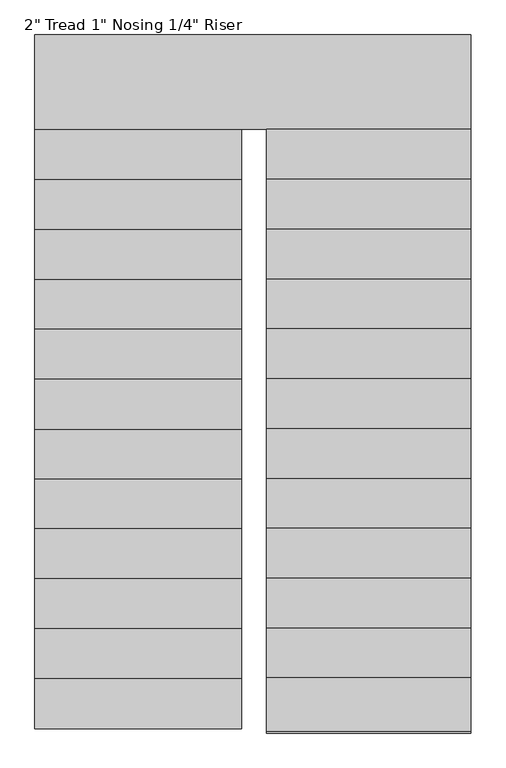
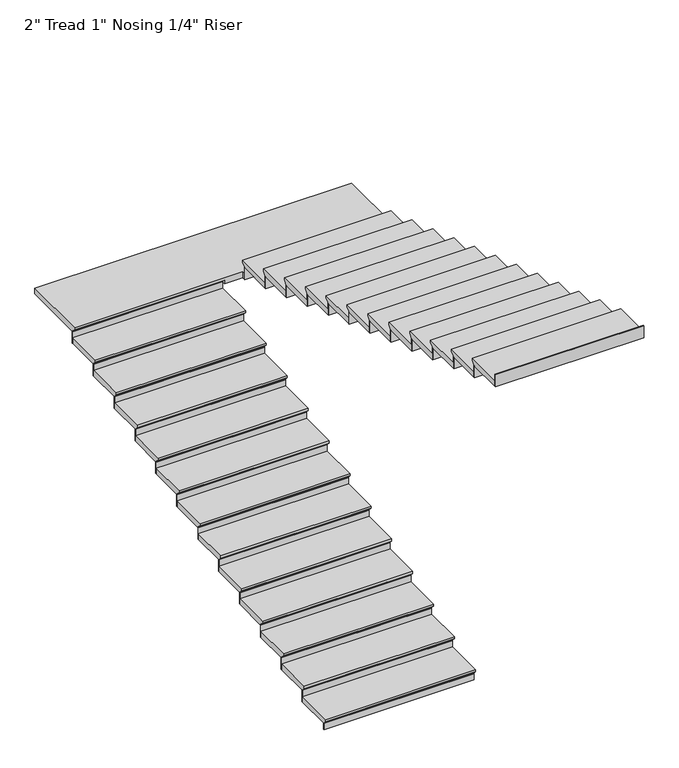
"""IFC4 building model written with IfcOpenShell, lengths in millimetres: stair flight geometry."""

from ifc_helpers import new_model, si_unit, origin, place, context, project, spatial, faceted_brep, source, transform, mapped, element, save


def stair_flight_b14bcda7(model_context):
    return source(origin(), model_context, "Body", "Brep", [
        faceted_brep([(-2593.7381751, -9955.5916506, 6182.4576923), (-2593.7381751, -9955.5916506, 6201.5076923), (-3857.687215, -9955.5916506, 6201.5076923), (-3857.687215, -9955.5916506, 6182.4576923), (-2593.7381751, -9930.1916506, 6157.0576923), (-3857.687215, -9930.1916506, 6157.0576923), (-2593.7381751, -9619.0416506, 6201.5076923), (-3857.687215, -9619.0416506, 6201.5076923), (-3857.687215, -9930.1916506, 6150.7076923), (-3857.687215, -9619.0416506, 6150.7076923), (-2593.7381751, -9619.0416506, 6150.7076923), (-2593.7381751, -9930.1916506, 6150.7076923)], [[[0, 1, 2, 3]], [[4, 0, 3, 5]], [[2, 1, 6, 7]], [[8, 9, 10, 11]], [[2, 7, 9, 8, 5, 3]], [[8, 11, 4, 5]], [[6, 1, 0, 4, 11, 10]], [[7, 6, 10, 9]]]),
        faceted_brep([(-2593.7381751, -9930.1916506, 6150.7076923), (-2593.7381751, -9930.1916506, 6096.0), (-2593.7381751, -9923.8416506, 6096.0), (-2593.7381751, -9923.8416506, 6150.7076923), (-3857.687215, -9930.1916506, 6150.7076923), (-3857.687215, -9923.8416506, 6150.7076923), (-3857.687215, -9923.8416506, 6096.0), (-3857.687215, -9930.1916506, 6096.0)], [[[0, 1, 2, 3]], [[4, 5, 6, 7]], [[1, 0, 4, 7]], [[2, 1, 7, 6]], [[3, 2, 6, 5]], [[0, 3, 5, 4]]]),
        faceted_brep([(-2593.7381751, -9619.0416506, 6256.2153846), (-2593.7381751, -9619.0416506, 6150.7076923), (-2593.7381751, -9612.6916506, 6150.7076923), (-2593.7381751, -9612.6916506, 6256.2153846), (-3857.687215, -9619.0416506, 6256.2153846), (-3857.687215, -9612.6916506, 6256.2153846), (-3857.687215, -9612.6916506, 6150.7076923), (-3857.687215, -9619.0416506, 6150.7076923)], [[[0, 1, 2, 3]], [[4, 5, 6, 7]], [[1, 0, 4, 7]], [[2, 1, 7, 6]], [[3, 2, 6, 5]], [[0, 3, 5, 4]]]),
        faceted_brep([(-3857.687215, -9644.4416506, 6307.0153846), (-2593.7381751, -9644.4416506, 6307.0153846), (-2593.7381751, -9314.2416506, 6307.0153846), (-3857.687215, -9314.2416506, 6307.0153846), (-3857.687215, -9619.0416506, 6256.2153846), (-3857.687215, -9314.2416506, 6256.2153846), (-2593.7381751, -9314.2416506, 6256.2153846), (-2593.7381751, -9619.0416506, 6256.2153846), (-3857.687215, -9619.0416506, 6262.5653846), (-3857.687215, -9644.4416506, 6287.9653846), (-2593.7381751, -9619.0416506, 6262.5653846), (-2593.7381751, -9644.4416506, 6287.9653846)], [[[0, 1, 2, 3]], [[4, 5, 6, 7]], [[0, 3, 5, 4, 8, 9]], [[4, 7, 10, 8]], [[2, 1, 11, 10, 7, 6]], [[3, 2, 6, 5]], [[11, 1, 0, 9]], [[10, 11, 9, 8]]]),
        faceted_brep([(-2593.7381751, -9314.2416506, 6361.7230769), (-2593.7381751, -9314.2416506, 6256.2153846), (-2593.7381751, -9307.8916506, 6256.2153846), (-2593.7381751, -9307.8916506, 6361.7230769), (-3857.687215, -9314.2416506, 6361.7230769), (-3857.687215, -9307.8916506, 6361.7230769), (-3857.687215, -9307.8916506, 6256.2153846), (-3857.687215, -9314.2416506, 6256.2153846)], [[[0, 1, 2, 3]], [[4, 5, 6, 7]], [[1, 0, 4, 7]], [[2, 1, 7, 6]], [[3, 2, 6, 5]], [[0, 3, 5, 4]]]),
        faceted_brep([(-3857.687215, -9339.6416506, 6412.5230769), (-2593.7381751, -9339.6416506, 6412.5230769), (-2593.7381751, -9009.4416506, 6412.5230769), (-3857.687215, -9009.4416506, 6412.5230769), (-3857.687215, -9314.2416506, 6361.7230769), (-3857.687215, -9009.4416506, 6361.7230769), (-2593.7381751, -9009.4416506, 6361.7230769), (-2593.7381751, -9314.2416506, 6361.7230769), (-3857.687215, -9314.2416506, 6368.0730769), (-3857.687215, -9339.6416506, 6393.4730769), (-2593.7381751, -9314.2416506, 6368.0730769), (-2593.7381751, -9339.6416506, 6393.4730769)], [[[0, 1, 2, 3]], [[4, 5, 6, 7]], [[0, 3, 5, 4, 8, 9]], [[4, 7, 10, 8]], [[2, 1, 11, 10, 7, 6]], [[3, 2, 6, 5]], [[11, 1, 0, 9]], [[10, 11, 9, 8]]]),
        faceted_brep([(-2593.7381751, -9009.4416506, 6467.2307692), (-2593.7381751, -9009.4416506, 6361.7230769), (-2593.7381751, -9003.0916506, 6361.7230769), (-2593.7381751, -9003.0916506, 6467.2307692), (-3857.687215, -9009.4416506, 6467.2307692), (-3857.687215, -9003.0916506, 6467.2307692), (-3857.687215, -9003.0916506, 6361.7230769), (-3857.687215, -9009.4416506, 6361.7230769)], [[[0, 1, 2, 3]], [[4, 5, 6, 7]], [[1, 0, 4, 7]], [[2, 1, 7, 6]], [[3, 2, 6, 5]], [[0, 3, 5, 4]]]),
        faceted_brep([(-3857.687215, -9034.8416506, 6518.0307692), (-2593.7381751, -9034.8416506, 6518.0307692), (-2593.7381751, -8704.6416506, 6518.0307692), (-3857.687215, -8704.6416506, 6518.0307692), (-3857.687215, -9009.4416506, 6467.2307692), (-3857.687215, -8704.6416506, 6467.2307692), (-2593.7381751, -8704.6416506, 6467.2307692), (-2593.7381751, -9009.4416506, 6467.2307692), (-3857.687215, -9009.4416506, 6473.5807692), (-3857.687215, -9034.8416506, 6498.9807692), (-2593.7381751, -9009.4416506, 6473.5807692), (-2593.7381751, -9034.8416506, 6498.9807692)], [[[0, 1, 2, 3]], [[4, 5, 6, 7]], [[0, 3, 5, 4, 8, 9]], [[4, 7, 10, 8]], [[2, 1, 11, 10, 7, 6]], [[3, 2, 6, 5]], [[11, 1, 0, 9]], [[10, 11, 9, 8]]]),
        faceted_brep([(-2593.7381751, -8704.6416506, 6572.7384615), (-2593.7381751, -8704.6416506, 6467.2307692), (-2593.7381751, -8698.2916506, 6467.2307692), (-2593.7381751, -8698.2916506, 6572.7384615), (-3857.687215, -8704.6416506, 6572.7384615), (-3857.687215, -8698.2916506, 6572.7384615), (-3857.687215, -8698.2916506, 6467.2307692), (-3857.687215, -8704.6416506, 6467.2307692)], [[[0, 1, 2, 3]], [[4, 5, 6, 7]], [[1, 0, 4, 7]], [[2, 1, 7, 6]], [[3, 2, 6, 5]], [[0, 3, 5, 4]]]),
        faceted_brep([(-3857.687215, -8730.0416506, 6623.5384615), (-2593.7381751, -8730.0416506, 6623.5384615), (-2593.7381751, -8399.8416506, 6623.5384615), (-3857.687215, -8399.8416506, 6623.5384615), (-3857.687215, -8704.6416506, 6572.7384615), (-3857.687215, -8399.8416506, 6572.7384615), (-2593.7381751, -8399.8416506, 6572.7384615), (-2593.7381751, -8704.6416506, 6572.7384615), (-3857.687215, -8704.6416506, 6579.0884615), (-3857.687215, -8730.0416506, 6604.4884615), (-2593.7381751, -8704.6416506, 6579.0884615), (-2593.7381751, -8730.0416506, 6604.4884615)], [[[0, 1, 2, 3]], [[4, 5, 6, 7]], [[0, 3, 5, 4, 8, 9]], [[4, 7, 10, 8]], [[2, 1, 11, 10, 7, 6]], [[3, 2, 6, 5]], [[11, 1, 0, 9]], [[10, 11, 9, 8]]]),
        faceted_brep([(-2593.7381751, -8399.8416506, 6678.2461538), (-2593.7381751, -8399.8416506, 6572.7384615), (-2593.7381751, -8393.4916506, 6572.7384615), (-2593.7381751, -8393.4916506, 6678.2461538), (-3857.687215, -8399.8416506, 6678.2461538), (-3857.687215, -8393.4916506, 6678.2461538), (-3857.687215, -8393.4916506, 6572.7384615), (-3857.687215, -8399.8416506, 6572.7384615)], [[[0, 1, 2, 3]], [[4, 5, 6, 7]], [[1, 0, 4, 7]], [[2, 1, 7, 6]], [[3, 2, 6, 5]], [[0, 3, 5, 4]]]),
        faceted_brep([(-3857.687215, -8425.2416506, 6729.0461538), (-2593.7381751, -8425.2416506, 6729.0461538), (-2593.7381751, -8098.2166506, 6729.0461538), (-3857.687215, -8098.2166506, 6729.0461538), (-3857.687215, -8399.8416506, 6678.2461538), (-3857.687215, -8098.2166506, 6678.2461538), (-2593.7381751, -8098.2166506, 6678.2461538), (-2593.7381751, -8399.8416506, 6678.2461538), (-3857.687215, -8399.8416506, 6684.5961538), (-3857.687215, -8425.2416506, 6709.9961538), (-2593.7381751, -8399.8416506, 6684.5961538), (-2593.7381751, -8425.2416506, 6709.9961538)], [[[0, 1, 2, 3]], [[4, 5, 6, 7]], [[0, 3, 5, 4, 8, 9]], [[4, 7, 10, 8]], [[2, 1, 11, 10, 7, 6]], [[3, 2, 6, 5]], [[11, 1, 0, 9]], [[10, 11, 9, 8]]]),
        faceted_brep([(-2593.7381751, -8098.2166506, 6783.7538462), (-2593.7381751, -8098.2166506, 6678.2461538), (-2593.7381751, -8091.8666506, 6678.2461538), (-2593.7381751, -8091.8666506, 6783.7538462), (-3857.687215, -8098.2166506, 6783.7538462), (-3857.687215, -8091.8666506, 6783.7538462), (-3857.687215, -8091.8666506, 6678.2461538), (-3857.687215, -8098.2166506, 6678.2461538)], [[[0, 1, 2, 3]], [[4, 5, 6, 7]], [[1, 0, 4, 7]], [[2, 1, 7, 6]], [[3, 2, 6, 5]], [[0, 3, 5, 4]]]),
        faceted_brep([(-3857.687215, -8123.6166506, 6834.5538462), (-2593.7381751, -8123.6166506, 6834.5538462), (-2593.7381751, -7790.2416506, 6834.5538462), (-3857.687215, -7790.2416506, 6834.5538462), (-3857.687215, -8098.2166506, 6783.7538462), (-3857.687215, -7790.2416506, 6783.7538462), (-2593.7381751, -7790.2416506, 6783.7538462), (-2593.7381751, -8098.2166506, 6783.7538462), (-3857.687215, -8098.2166506, 6790.1038462), (-3857.687215, -8123.6166506, 6815.5038462), (-2593.7381751, -8098.2166506, 6790.1038462), (-2593.7381751, -8123.6166506, 6815.5038462)], [[[0, 1, 2, 3]], [[4, 5, 6, 7]], [[0, 3, 5, 4, 8, 9]], [[4, 7, 10, 8]], [[2, 1, 11, 10, 7, 6]], [[3, 2, 6, 5]], [[11, 1, 0, 9]], [[10, 11, 9, 8]]]),
        faceted_brep([(-2593.7381751, -7790.2416506, 6889.2615385), (-2593.7381751, -7790.2416506, 6783.7538462), (-2593.7381751, -7783.8916506, 6783.7538462), (-2593.7381751, -7783.8916506, 6889.2615385), (-3857.687215, -7790.2416506, 6889.2615385), (-3857.687215, -7783.8916506, 6889.2615385), (-3857.687215, -7783.8916506, 6783.7538462), (-3857.687215, -7790.2416506, 6783.7538462)], [[[0, 1, 2, 3]], [[4, 5, 6, 7]], [[1, 0, 4, 7]], [[2, 1, 7, 6]], [[3, 2, 6, 5]], [[0, 3, 5, 4]]]),
        faceted_brep([(-3857.687215, -7815.6416506, 6940.0615385), (-2593.7381751, -7815.6416506, 6940.0615385), (-2593.7381751, -7485.4416506, 6940.0615385), (-3857.687215, -7485.4416506, 6940.0615385), (-3857.687215, -7790.2416506, 6889.2615385), (-3857.687215, -7485.4416506, 6889.2615385), (-2593.7381751, -7485.4416506, 6889.2615385), (-2593.7381751, -7790.2416506, 6889.2615385), (-3857.687215, -7790.2416506, 6895.6115385), (-3857.687215, -7815.6416506, 6921.0115385), (-2593.7381751, -7790.2416506, 6895.6115385), (-2593.7381751, -7815.6416506, 6921.0115385)], [[[0, 1, 2, 3]], [[4, 5, 6, 7]], [[0, 3, 5, 4, 8, 9]], [[4, 7, 10, 8]], [[2, 1, 11, 10, 7, 6]], [[3, 2, 6, 5]], [[11, 1, 0, 9]], [[10, 11, 9, 8]]]),
        faceted_brep([(-2593.7381751, -7485.4416506, 6994.7692308), (-2593.7381751, -7485.4416506, 6889.2615385), (-2593.7381751, -7479.0916506, 6889.2615385), (-2593.7381751, -7479.0916506, 6994.7692308), (-3857.687215, -7485.4416506, 6994.7692308), (-3857.687215, -7479.0916506, 6994.7692308), (-3857.687215, -7479.0916506, 6889.2615385), (-3857.687215, -7485.4416506, 6889.2615385)], [[[0, 1, 2, 3]], [[4, 5, 6, 7]], [[1, 0, 4, 7]], [[2, 1, 7, 6]], [[3, 2, 6, 5]], [[0, 3, 5, 4]]]),
        faceted_brep([(-3857.687215, -7510.8416506, 7045.5692308), (-2593.7381751, -7510.8416506, 7045.5692308), (-2593.7381751, -7180.6416506, 7045.5692308), (-3857.687215, -7180.6416506, 7045.5692308), (-3857.687215, -7485.4416506, 6994.7692308), (-3857.687215, -7180.6416506, 6994.7692308), (-2593.7381751, -7180.6416506, 6994.7692308), (-2593.7381751, -7485.4416506, 6994.7692308), (-3857.687215, -7485.4416506, 7001.1192308), (-3857.687215, -7510.8416506, 7026.5192308), (-2593.7381751, -7485.4416506, 7001.1192308), (-2593.7381751, -7510.8416506, 7026.5192308)], [[[0, 1, 2, 3]], [[4, 5, 6, 7]], [[0, 3, 5, 4, 8, 9]], [[4, 7, 10, 8]], [[2, 1, 11, 10, 7, 6]], [[3, 2, 6, 5]], [[11, 1, 0, 9]], [[10, 11, 9, 8]]]),
        faceted_brep([(-2593.7381751, -7180.6416506, 7100.2769231), (-2593.7381751, -7180.6416506, 6994.7692308), (-2593.7381751, -7174.2916506, 6994.7692308), (-2593.7381751, -7174.2916506, 7100.2769231), (-3857.687215, -7180.6416506, 7100.2769231), (-3857.687215, -7174.2916506, 7100.2769231), (-3857.687215, -7174.2916506, 6994.7692308), (-3857.687215, -7180.6416506, 6994.7692308)], [[[0, 1, 2, 3]], [[4, 5, 6, 7]], [[1, 0, 4, 7]], [[2, 1, 7, 6]], [[3, 2, 6, 5]], [[0, 3, 5, 4]]]),
        faceted_brep([(-3857.687215, -7206.0416506, 7151.0769231), (-2593.7381751, -7206.0416506, 7151.0769231), (-2593.7381751, -6875.8416506, 7151.0769231), (-3857.687215, -6875.8416506, 7151.0769231), (-3857.687215, -7180.6416506, 7100.2769231), (-3857.687215, -6875.8416506, 7100.2769231), (-2593.7381751, -6875.8416506, 7100.2769231), (-2593.7381751, -7180.6416506, 7100.2769231), (-3857.687215, -7180.6416506, 7106.6269231), (-3857.687215, -7206.0416506, 7132.0269231), (-2593.7381751, -7180.6416506, 7106.6269231), (-2593.7381751, -7206.0416506, 7132.0269231)], [[[0, 1, 2, 3]], [[4, 5, 6, 7]], [[0, 3, 5, 4, 8, 9]], [[4, 7, 10, 8]], [[2, 1, 11, 10, 7, 6]], [[3, 2, 6, 5]], [[11, 1, 0, 9]], [[10, 11, 9, 8]]]),
        faceted_brep([(-2593.7381751, -6875.8416506, 7205.7846154), (-2593.7381751, -6875.8416506, 7100.2769231), (-2593.7381751, -6869.4916506, 7100.2769231), (-2593.7381751, -6869.4916506, 7205.7846154), (-3857.687215, -6875.8416506, 7205.7846154), (-3857.687215, -6869.4916506, 7205.7846154), (-3857.687215, -6869.4916506, 7100.2769231), (-3857.687215, -6875.8416506, 7100.2769231)], [[[0, 1, 2, 3]], [[4, 5, 6, 7]], [[1, 0, 4, 7]], [[2, 1, 7, 6]], [[3, 2, 6, 5]], [[0, 3, 5, 4]]]),
        faceted_brep([(-3857.687215, -6901.2416506, 7256.5846154), (-2593.7381751, -6901.2416506, 7256.5846154), (-2593.7381751, -6571.0416506, 7256.5846154), (-3857.687215, -6571.0416506, 7256.5846154), (-3857.687215, -6875.8416506, 7205.7846154), (-3857.687215, -6571.0416506, 7205.7846154), (-2593.7381751, -6571.0416506, 7205.7846154), (-2593.7381751, -6875.8416506, 7205.7846154), (-3857.687215, -6875.8416506, 7212.1346154), (-3857.687215, -6901.2416506, 7237.5346154), (-2593.7381751, -6875.8416506, 7212.1346154), (-2593.7381751, -6901.2416506, 7237.5346154)], [[[0, 1, 2, 3]], [[4, 5, 6, 7]], [[0, 3, 5, 4, 8, 9]], [[4, 7, 10, 8]], [[2, 1, 11, 10, 7, 6]], [[3, 2, 6, 5]], [[11, 1, 0, 9]], [[10, 11, 9, 8]]]),
        faceted_brep([(-2593.7381751, -6571.0416506, 7311.2923077), (-2593.7381751, -6571.0416506, 7205.7846154), (-2593.7381751, -6564.6916506, 7205.7846154), (-2593.7381751, -6564.6916506, 7311.2923077), (-3857.687215, -6571.0416506, 7311.2923077), (-3857.687215, -6564.6916506, 7311.2923077), (-3857.687215, -6564.6916506, 7205.7846154), (-3857.687215, -6571.0416506, 7205.7846154)], [[[0, 1, 2, 3]], [[4, 5, 6, 7]], [[1, 0, 4, 7]], [[2, 1, 7, 6]], [[3, 2, 6, 5]], [[0, 3, 5, 4]]]),
        faceted_brep([(-3857.687215, -6596.4416506, 7362.0923077), (-2593.7381751, -6596.4416506, 7362.0923077), (-2593.7381751, -6266.2416506, 7362.0923077), (-3857.687215, -6266.2416506, 7362.0923077), (-3857.687215, -6571.0416506, 7311.2923077), (-3857.687215, -6266.2416506, 7311.2923077), (-2593.7381751, -6266.2416506, 7311.2923077), (-2593.7381751, -6571.0416506, 7311.2923077), (-3857.687215, -6571.0416506, 7317.6423077), (-3857.687215, -6596.4416506, 7343.0423077), (-2593.7381751, -6571.0416506, 7317.6423077), (-2593.7381751, -6596.4416506, 7343.0423077)], [[[0, 1, 2, 3]], [[4, 5, 6, 7]], [[0, 3, 5, 4, 8, 9]], [[4, 7, 10, 8]], [[2, 1, 11, 10, 7, 6]], [[3, 2, 6, 5]], [[11, 1, 0, 9]], [[10, 11, 9, 8]]]),
        faceted_brep([(-2593.7381751, -6266.2416506, 7416.8), (-2593.7381751, -6266.2416506, 7311.2923077), (-2593.7381751, -6259.8916506, 7311.2923077), (-2593.7381751, -6259.8916506, 7416.8), (-3857.687215, -6266.2416506, 7416.8), (-3857.687215, -6259.8916506, 7416.8), (-3857.687215, -6259.8916506, 7311.2923077), (-3857.687215, -6266.2416506, 7311.2923077)], [[[0, 1, 2, 3]], [[4, 5, 6, 7]], [[1, 0, 4, 7]], [[2, 1, 7, 6]], [[3, 2, 6, 5]], [[0, 3, 5, 4]]]),
        faceted_brep([(-1190.687215, -6317.0416506, 7467.6), (-1190.687215, -5713.7916506, 7467.6), (-3857.687215, -5713.7916506, 7467.6), (-3857.687215, -6291.6416506, 7467.6), (-2441.3381751, -6291.6416506, 7467.6), (-2441.3381751, -6317.0416506, 7467.6), (-1190.687215, -5713.7916506, 7416.8), (-1190.687215, -6317.0416506, 7416.8), (-2441.3381751, -6317.0416506, 7416.8), (-2441.3381751, -6291.6416506, 7416.8), (-2593.7381751, -6291.6416506, 7416.8), (-2593.7381751, -6266.2416506, 7416.8), (-3857.687215, -6266.2416506, 7416.8), (-3857.687215, -5713.7916506, 7416.8), (-3857.687215, -6266.2416506, 7423.15), (-3857.687215, -6291.6416506, 7448.55), (-2593.7381751, -6266.2416506, 7423.15), (-2593.7381751, -6291.6416506, 7448.55)], [[[0, 1, 2, 3, 4, 5]], [[6, 7, 8, 9, 10, 11, 12, 13]], [[1, 0, 7, 6]], [[2, 1, 6, 13]], [[3, 2, 13, 12, 14, 15]], [[12, 11, 16, 14]], [[11, 10, 17, 16]], [[4, 3, 15, 17, 10, 9]], [[5, 4, 9, 8]], [[0, 5, 8, 7]], [[15, 14, 16, 17]]]),
        faceted_brep([(-2441.3381751, -6317.0416506, 7522.3076923), (-2441.3381751, -6317.0416506, 7416.8), (-2441.3381751, -6323.3916506, 7416.8), (-2441.3381751, -6323.3916506, 7522.3076923), (-1190.687215, -6317.0416506, 7522.3076923), (-1190.687215, -6323.3916506, 7522.3076923), (-1190.687215, -6323.3916506, 7416.8), (-1190.687215, -6317.0416506, 7416.8)], [[[0, 1, 2, 3]], [[4, 5, 6, 7]], [[1, 0, 4, 7]], [[2, 1, 7, 6]], [[3, 2, 6, 5]], [[0, 3, 5, 4]]]),
        faceted_brep([(-1190.687215, -6291.6416506, 7573.1076923), (-2441.3381751, -6291.6416506, 7573.1076923), (-2441.3381751, -6621.8416506, 7573.1076923), (-1190.687215, -6621.8416506, 7573.1076923), (-1190.687215, -6317.0416506, 7522.3076923), (-1190.687215, -6621.8416506, 7522.3076923), (-2441.3381751, -6621.8416506, 7522.3076923), (-2441.3381751, -6317.0416506, 7522.3076923), (-1190.687215, -6317.0416506, 7528.6576923), (-1190.687215, -6291.6416506, 7554.0576923), (-2441.3381751, -6317.0416506, 7528.6576923), (-2441.3381751, -6291.6416506, 7554.0576923)], [[[0, 1, 2, 3]], [[4, 5, 6, 7]], [[0, 3, 5, 4, 8, 9]], [[4, 7, 10, 8]], [[2, 1, 11, 10, 7, 6]], [[3, 2, 6, 5]], [[11, 1, 0, 9]], [[10, 11, 9, 8]]]),
        faceted_brep([(-2441.3381751, -6621.8416506, 7627.8153846), (-2441.3381751, -6621.8416506, 7522.3076923), (-2441.3381751, -6628.1916506, 7522.3076923), (-2441.3381751, -6628.1916506, 7627.8153846), (-1190.687215, -6621.8416506, 7627.8153846), (-1190.687215, -6628.1916506, 7627.8153846), (-1190.687215, -6628.1916506, 7522.3076923), (-1190.687215, -6621.8416506, 7522.3076923)], [[[0, 1, 2, 3]], [[4, 5, 6, 7]], [[1, 0, 4, 7]], [[2, 1, 7, 6]], [[3, 2, 6, 5]], [[0, 3, 5, 4]]]),
        faceted_brep([(-1190.687215, -6596.4416506, 7678.6153846), (-2441.3381751, -6596.4416506, 7678.6153846), (-2441.3381751, -6926.6416506, 7678.6153846), (-1190.687215, -6926.6416506, 7678.6153846), (-1190.687215, -6621.8416506, 7627.8153846), (-1190.687215, -6926.6416506, 7627.8153846), (-2441.3381751, -6926.6416506, 7627.8153846), (-2441.3381751, -6621.8416506, 7627.8153846), (-1190.687215, -6621.8416506, 7634.1653846), (-1190.687215, -6596.4416506, 7659.5653846), (-2441.3381751, -6621.8416506, 7634.1653846), (-2441.3381751, -6596.4416506, 7659.5653846)], [[[0, 1, 2, 3]], [[4, 5, 6, 7]], [[0, 3, 5, 4, 8, 9]], [[4, 7, 10, 8]], [[2, 1, 11, 10, 7, 6]], [[3, 2, 6, 5]], [[11, 1, 0, 9]], [[10, 11, 9, 8]]]),
        faceted_brep([(-2441.3381751, -6926.6416506, 7733.3230769), (-2441.3381751, -6926.6416506, 7627.8153846), (-2441.3381751, -6932.9916506, 7627.8153846), (-2441.3381751, -6932.9916506, 7733.3230769), (-1190.687215, -6926.6416506, 7733.3230769), (-1190.687215, -6932.9916506, 7733.3230769), (-1190.687215, -6932.9916506, 7627.8153846), (-1190.687215, -6926.6416506, 7627.8153846)], [[[0, 1, 2, 3]], [[4, 5, 6, 7]], [[1, 0, 4, 7]], [[2, 1, 7, 6]], [[3, 2, 6, 5]], [[0, 3, 5, 4]]]),
        faceted_brep([(-1190.687215, -6901.2416506, 7784.1230769), (-2441.3381751, -6901.2416506, 7784.1230769), (-2441.3381751, -7231.4416506, 7784.1230769), (-1190.687215, -7231.4416506, 7784.1230769), (-1190.687215, -6926.6416506, 7733.3230769), (-1190.687215, -7231.4416506, 7733.3230769), (-2441.3381751, -7231.4416506, 7733.3230769), (-2441.3381751, -6926.6416506, 7733.3230769), (-1190.687215, -6926.6416506, 7739.6730769), (-1190.687215, -6901.2416506, 7765.0730769), (-2441.3381751, -6926.6416506, 7739.6730769), (-2441.3381751, -6901.2416506, 7765.0730769)], [[[0, 1, 2, 3]], [[4, 5, 6, 7]], [[0, 3, 5, 4, 8, 9]], [[4, 7, 10, 8]], [[2, 1, 11, 10, 7, 6]], [[3, 2, 6, 5]], [[11, 1, 0, 9]], [[10, 11, 9, 8]]]),
        faceted_brep([(-2441.3381751, -7231.4416506, 7838.8307692), (-2441.3381751, -7231.4416506, 7733.3230769), (-2441.3381751, -7237.7916506, 7733.3230769), (-2441.3381751, -7237.7916506, 7838.8307692), (-1190.687215, -7231.4416506, 7838.8307692), (-1190.687215, -7237.7916506, 7838.8307692), (-1190.687215, -7237.7916506, 7733.3230769), (-1190.687215, -7231.4416506, 7733.3230769)], [[[0, 1, 2, 3]], [[4, 5, 6, 7]], [[1, 0, 4, 7]], [[2, 1, 7, 6]], [[3, 2, 6, 5]], [[0, 3, 5, 4]]]),
        faceted_brep([(-1190.687215, -7206.0416506, 7889.6307692), (-2441.3381751, -7206.0416506, 7889.6307692), (-2441.3381751, -7536.2416506, 7889.6307692), (-1190.687215, -7536.2416506, 7889.6307692), (-1190.687215, -7231.4416506, 7838.8307692), (-1190.687215, -7536.2416506, 7838.8307692), (-2441.3381751, -7536.2416506, 7838.8307692), (-2441.3381751, -7231.4416506, 7838.8307692), (-1190.687215, -7231.4416506, 7845.1807692), (-1190.687215, -7206.0416506, 7870.5807692), (-2441.3381751, -7231.4416506, 7845.1807692), (-2441.3381751, -7206.0416506, 7870.5807692)], [[[0, 1, 2, 3]], [[4, 5, 6, 7]], [[0, 3, 5, 4, 8, 9]], [[4, 7, 10, 8]], [[2, 1, 11, 10, 7, 6]], [[3, 2, 6, 5]], [[11, 1, 0, 9]], [[10, 11, 9, 8]]]),
        faceted_brep([(-2441.3381751, -7536.2416506, 7944.3384615), (-2441.3381751, -7536.2416506, 7838.8307692), (-2441.3381751, -7542.5916506, 7838.8307692), (-2441.3381751, -7542.5916506, 7944.3384615), (-1190.687215, -7536.2416506, 7944.3384615), (-1190.687215, -7542.5916506, 7944.3384615), (-1190.687215, -7542.5916506, 7838.8307692), (-1190.687215, -7536.2416506, 7838.8307692)], [[[0, 1, 2, 3]], [[4, 5, 6, 7]], [[1, 0, 4, 7]], [[2, 1, 7, 6]], [[3, 2, 6, 5]], [[0, 3, 5, 4]]]),
        faceted_brep([(-1190.687215, -7510.8416506, 7995.1384615), (-2441.3381751, -7510.8416506, 7995.1384615), (-2441.3381751, -7841.0416506, 7995.1384615), (-1190.687215, -7841.0416506, 7995.1384615), (-1190.687215, -7536.2416506, 7944.3384615), (-1190.687215, -7841.0416506, 7944.3384615), (-2441.3381751, -7841.0416506, 7944.3384615), (-2441.3381751, -7536.2416506, 7944.3384615), (-1190.687215, -7536.2416506, 7950.6884615), (-1190.687215, -7510.8416506, 7976.0884615), (-2441.3381751, -7536.2416506, 7950.6884615), (-2441.3381751, -7510.8416506, 7976.0884615)], [[[0, 1, 2, 3]], [[4, 5, 6, 7]], [[0, 3, 5, 4, 8, 9]], [[4, 7, 10, 8]], [[2, 1, 11, 10, 7, 6]], [[3, 2, 6, 5]], [[11, 1, 0, 9]], [[10, 11, 9, 8]]]),
        faceted_brep([(-2441.3381751, -7841.0416506, 8049.8461538), (-2441.3381751, -7841.0416506, 7944.3384615), (-2441.3381751, -7847.3916506, 7944.3384615), (-2441.3381751, -7847.3916506, 8049.8461538), (-1190.687215, -7841.0416506, 8049.8461538), (-1190.687215, -7847.3916506, 8049.8461538), (-1190.687215, -7847.3916506, 7944.3384615), (-1190.687215, -7841.0416506, 7944.3384615)], [[[0, 1, 2, 3]], [[4, 5, 6, 7]], [[1, 0, 4, 7]], [[2, 1, 7, 6]], [[3, 2, 6, 5]], [[0, 3, 5, 4]]]),
        faceted_brep([(-1190.687215, -7815.6416506, 8100.6461538), (-2441.3381751, -7815.6416506, 8100.6461538), (-2441.3381751, -8145.8416506, 8100.6461538), (-1190.687215, -8145.8416506, 8100.6461538), (-1190.687215, -7841.0416506, 8049.8461538), (-1190.687215, -8145.8416506, 8049.8461538), (-2441.3381751, -8145.8416506, 8049.8461538), (-2441.3381751, -7841.0416506, 8049.8461538), (-1190.687215, -7841.0416506, 8056.1961538), (-1190.687215, -7815.6416506, 8081.5961538), (-2441.3381751, -7841.0416506, 8056.1961538), (-2441.3381751, -7815.6416506, 8081.5961538)], [[[0, 1, 2, 3]], [[4, 5, 6, 7]], [[0, 3, 5, 4, 8, 9]], [[4, 7, 10, 8]], [[2, 1, 11, 10, 7, 6]], [[3, 2, 6, 5]], [[11, 1, 0, 9]], [[10, 11, 9, 8]]]),
        faceted_brep([(-2441.3381751, -8145.8416506, 8155.3538462), (-2441.3381751, -8145.8416506, 8049.8461538), (-2441.3381751, -8152.1916506, 8049.8461538), (-2441.3381751, -8152.1916506, 8155.3538462), (-1190.687215, -8145.8416506, 8155.3538462), (-1190.687215, -8152.1916506, 8155.3538462), (-1190.687215, -8152.1916506, 8049.8461538), (-1190.687215, -8145.8416506, 8049.8461538)], [[[0, 1, 2, 3]], [[4, 5, 6, 7]], [[1, 0, 4, 7]], [[2, 1, 7, 6]], [[3, 2, 6, 5]], [[0, 3, 5, 4]]]),
        faceted_brep([(-1190.687215, -8120.4416506, 8206.1538462), (-2441.3381751, -8120.4416506, 8206.1538462), (-2441.3381751, -8450.6416506, 8206.1538462), (-1190.687215, -8450.6416506, 8206.1538462), (-1190.687215, -8145.8416506, 8155.3538462), (-1190.687215, -8450.6416506, 8155.3538462), (-2441.3381751, -8450.6416506, 8155.3538462), (-2441.3381751, -8145.8416506, 8155.3538462), (-1190.687215, -8145.8416506, 8161.7038462), (-1190.687215, -8120.4416506, 8187.1038462), (-2441.3381751, -8145.8416506, 8161.7038462), (-2441.3381751, -8120.4416506, 8187.1038462)], [[[0, 1, 2, 3]], [[4, 5, 6, 7]], [[0, 3, 5, 4, 8, 9]], [[4, 7, 10, 8]], [[2, 1, 11, 10, 7, 6]], [[3, 2, 6, 5]], [[11, 1, 0, 9]], [[10, 11, 9, 8]]]),
        faceted_brep([(-2441.3381751, -8450.6416506, 8260.8615385), (-2441.3381751, -8450.6416506, 8155.3538462), (-2441.3381751, -8456.9916506, 8155.3538462), (-2441.3381751, -8456.9916506, 8260.8615385), (-1190.687215, -8450.6416506, 8260.8615385), (-1190.687215, -8456.9916506, 8260.8615385), (-1190.687215, -8456.9916506, 8155.3538462), (-1190.687215, -8450.6416506, 8155.3538462)], [[[0, 1, 2, 3]], [[4, 5, 6, 7]], [[1, 0, 4, 7]], [[2, 1, 7, 6]], [[3, 2, 6, 5]], [[0, 3, 5, 4]]]),
        faceted_brep([(-1190.687215, -8425.2416506, 8311.6615385), (-2441.3381751, -8425.2416506, 8311.6615385), (-2441.3381751, -8755.4416506, 8311.6615385), (-1190.687215, -8755.4416506, 8311.6615385), (-1190.687215, -8450.6416506, 8260.8615385), (-1190.687215, -8755.4416506, 8260.8615385), (-2441.3381751, -8755.4416506, 8260.8615385), (-2441.3381751, -8450.6416506, 8260.8615385), (-1190.687215, -8450.6416506, 8267.2115385), (-1190.687215, -8425.2416506, 8292.6115385), (-2441.3381751, -8450.6416506, 8267.2115385), (-2441.3381751, -8425.2416506, 8292.6115385)], [[[0, 1, 2, 3]], [[4, 5, 6, 7]], [[0, 3, 5, 4, 8, 9]], [[4, 7, 10, 8]], [[2, 1, 11, 10, 7, 6]], [[3, 2, 6, 5]], [[11, 1, 0, 9]], [[10, 11, 9, 8]]]),
        faceted_brep([(-2441.3381751, -8755.4416506, 8366.3692308), (-2441.3381751, -8755.4416506, 8260.8615385), (-2441.3381751, -8761.7916506, 8260.8615385), (-2441.3381751, -8761.7916506, 8366.3692308), (-1190.687215, -8755.4416506, 8366.3692308), (-1190.687215, -8761.7916506, 8366.3692308), (-1190.687215, -8761.7916506, 8260.8615385), (-1190.687215, -8755.4416506, 8260.8615385)], [[[0, 1, 2, 3]], [[4, 5, 6, 7]], [[1, 0, 4, 7]], [[2, 1, 7, 6]], [[3, 2, 6, 5]], [[0, 3, 5, 4]]]),
        faceted_brep([(-1190.687215, -8730.0416506, 8417.1692308), (-2441.3381751, -8730.0416506, 8417.1692308), (-2441.3381751, -9060.2416506, 8417.1692308), (-1190.687215, -9060.2416506, 8417.1692308), (-1190.687215, -8755.4416506, 8366.3692308), (-1190.687215, -9060.2416506, 8366.3692308), (-2441.3381751, -9060.2416506, 8366.3692308), (-2441.3381751, -8755.4416506, 8366.3692308), (-1190.687215, -8755.4416506, 8372.7192308), (-1190.687215, -8730.0416506, 8398.1192308), (-2441.3381751, -8755.4416506, 8372.7192308), (-2441.3381751, -8730.0416506, 8398.1192308)], [[[0, 1, 2, 3]], [[4, 5, 6, 7]], [[0, 3, 5, 4, 8, 9]], [[4, 7, 10, 8]], [[2, 1, 11, 10, 7, 6]], [[3, 2, 6, 5]], [[11, 1, 0, 9]], [[10, 11, 9, 8]]]),
        faceted_brep([(-2441.3381751, -9060.2416506, 8471.8769231), (-2441.3381751, -9060.2416506, 8366.3692308), (-2441.3381751, -9066.5916506, 8366.3692308), (-2441.3381751, -9066.5916506, 8471.8769231), (-1190.687215, -9060.2416506, 8471.8769231), (-1190.687215, -9066.5916506, 8471.8769231), (-1190.687215, -9066.5916506, 8366.3692308), (-1190.687215, -9060.2416506, 8366.3692308)], [[[0, 1, 2, 3]], [[4, 5, 6, 7]], [[1, 0, 4, 7]], [[2, 1, 7, 6]], [[3, 2, 6, 5]], [[0, 3, 5, 4]]]),
        faceted_brep([(-1190.687215, -9034.8416506, 8522.6769231), (-2441.3381751, -9034.8416506, 8522.6769231), (-2441.3381751, -9365.0416506, 8522.6769231), (-1190.687215, -9365.0416506, 8522.6769231), (-1190.687215, -9060.2416506, 8471.8769231), (-1190.687215, -9365.0416506, 8471.8769231), (-2441.3381751, -9365.0416506, 8471.8769231), (-2441.3381751, -9060.2416506, 8471.8769231), (-1190.687215, -9060.2416506, 8478.2269231), (-1190.687215, -9034.8416506, 8503.6269231), (-2441.3381751, -9060.2416506, 8478.2269231), (-2441.3381751, -9034.8416506, 8503.6269231)], [[[0, 1, 2, 3]], [[4, 5, 6, 7]], [[0, 3, 5, 4, 8, 9]], [[4, 7, 10, 8]], [[2, 1, 11, 10, 7, 6]], [[3, 2, 6, 5]], [[11, 1, 0, 9]], [[10, 11, 9, 8]]]),
        faceted_brep([(-2441.3381751, -9365.0416506, 8577.3846154), (-2441.3381751, -9365.0416506, 8471.8769231), (-2441.3381751, -9371.3916506, 8471.8769231), (-2441.3381751, -9371.3916506, 8577.3846154), (-1190.687215, -9365.0416506, 8577.3846154), (-1190.687215, -9371.3916506, 8577.3846154), (-1190.687215, -9371.3916506, 8471.8769231), (-1190.687215, -9365.0416506, 8471.8769231)], [[[0, 1, 2, 3]], [[4, 5, 6, 7]], [[1, 0, 4, 7]], [[2, 1, 7, 6]], [[3, 2, 6, 5]], [[0, 3, 5, 4]]]),
        faceted_brep([(-1190.687215, -9339.6416506, 8628.1846154), (-2441.3381751, -9339.6416506, 8628.1846154), (-2441.3381751, -9669.8416506, 8628.1846154), (-1190.687215, -9669.8416506, 8628.1846154), (-1190.687215, -9365.0416506, 8577.3846154), (-1190.687215, -9669.8416506, 8577.3846154), (-2441.3381751, -9669.8416506, 8577.3846154), (-2441.3381751, -9365.0416506, 8577.3846154), (-1190.687215, -9365.0416506, 8583.7346154), (-1190.687215, -9339.6416506, 8609.1346154), (-2441.3381751, -9365.0416506, 8583.7346154), (-2441.3381751, -9339.6416506, 8609.1346154)], [[[0, 1, 2, 3]], [[4, 5, 6, 7]], [[0, 3, 5, 4, 8, 9]], [[4, 7, 10, 8]], [[2, 1, 11, 10, 7, 6]], [[3, 2, 6, 5]], [[11, 1, 0, 9]], [[10, 11, 9, 8]]]),
        faceted_brep([(-2441.3381751, -9669.8416506, 8682.8923077), (-2441.3381751, -9669.8416506, 8577.3846154), (-2441.3381751, -9676.1916506, 8577.3846154), (-2441.3381751, -9676.1916506, 8682.8923077), (-1190.687215, -9669.8416506, 8682.8923077), (-1190.687215, -9676.1916506, 8682.8923077), (-1190.687215, -9676.1916506, 8577.3846154), (-1190.687215, -9669.8416506, 8577.3846154)], [[[0, 1, 2, 3]], [[4, 5, 6, 7]], [[1, 0, 4, 7]], [[2, 1, 7, 6]], [[3, 2, 6, 5]], [[0, 3, 5, 4]]]),
        faceted_brep([(-2441.3381751, -9974.6416506, 8788.4), (-2441.3381751, -9974.6416506, 8682.8923077), (-2441.3381751, -9980.9916506, 8682.8923077), (-2441.3381751, -9980.9916506, 8788.4), (-1190.687215, -9974.6416506, 8788.4), (-1190.687215, -9980.9916506, 8788.4), (-1190.687215, -9980.9916506, 8682.8923077), (-1190.687215, -9974.6416506, 8682.8923077)], [[[0, 1, 2, 3]], [[4, 5, 6, 7]], [[1, 0, 4, 7]], [[2, 1, 7, 6]], [[3, 2, 6, 5]], [[0, 3, 5, 4]]]),
        faceted_brep([(-1190.687215, -9644.4416506, 8733.6923077), (-2441.3381751, -9644.4416506, 8733.6923077), (-2441.3381751, -9974.6416506, 8733.6923077), (-1190.687215, -9974.6416506, 8733.6923077), (-1190.687215, -9669.8416506, 8682.8923077), (-1190.687215, -9974.6416506, 8682.8923077), (-2441.3381751, -9974.6416506, 8682.8923077), (-2441.3381751, -9669.8416506, 8682.8923077), (-1190.687215, -9669.8416506, 8689.2423077), (-1190.687215, -9644.4416506, 8714.6423077), (-2441.3381751, -9669.8416506, 8689.2423077), (-2441.3381751, -9644.4416506, 8714.6423077)], [[[0, 1, 2, 3]], [[4, 5, 6, 7]], [[0, 3, 5, 4, 8, 9]], [[4, 7, 10, 8]], [[2, 1, 11, 10, 7, 6]], [[3, 2, 6, 5]], [[11, 1, 0, 9]], [[10, 11, 9, 8]]]),
    ])


if __name__ == "__main__":
    model = new_model("IFC4")
    model_context = context("Model", 3, world=origin())
    ifc_project = project(units=[si_unit("LENGTHUNIT", "METRE", prefix="MILLI")], contexts=[model_context])
    site = spatial("IfcSite", under=ifc_project)
    building = spatial("IfcBuilding", under=site)
    placement = place(None, origin())
    stair_flight_shape = stair_flight_b14bcda7(model_context)
    element("IfcStairFlight", 1, ObjectType="2\" Tread 1\" Nosing 1/4\" Riser", at=placement, inside=building, context=model_context, shape_type="MappedRepresentation", body=[
        mapped(stair_flight_shape, transform((0.0, 0.0, 0.0), x_axis=(1.0, 0.0, 0.0), y_axis=(0.0, 1.0, 0.0), z_axis=(0.0, 0.0, 1.0))),
    ])
    save(model, "model.ifc")
